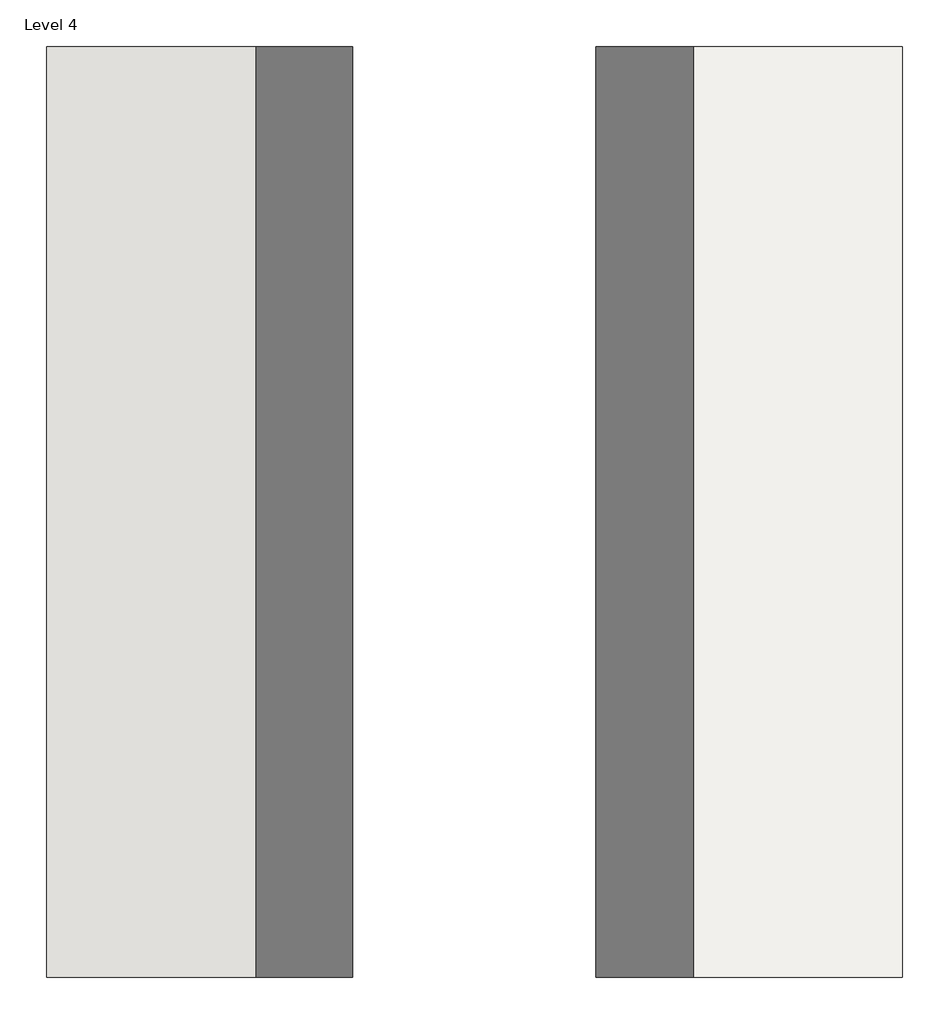
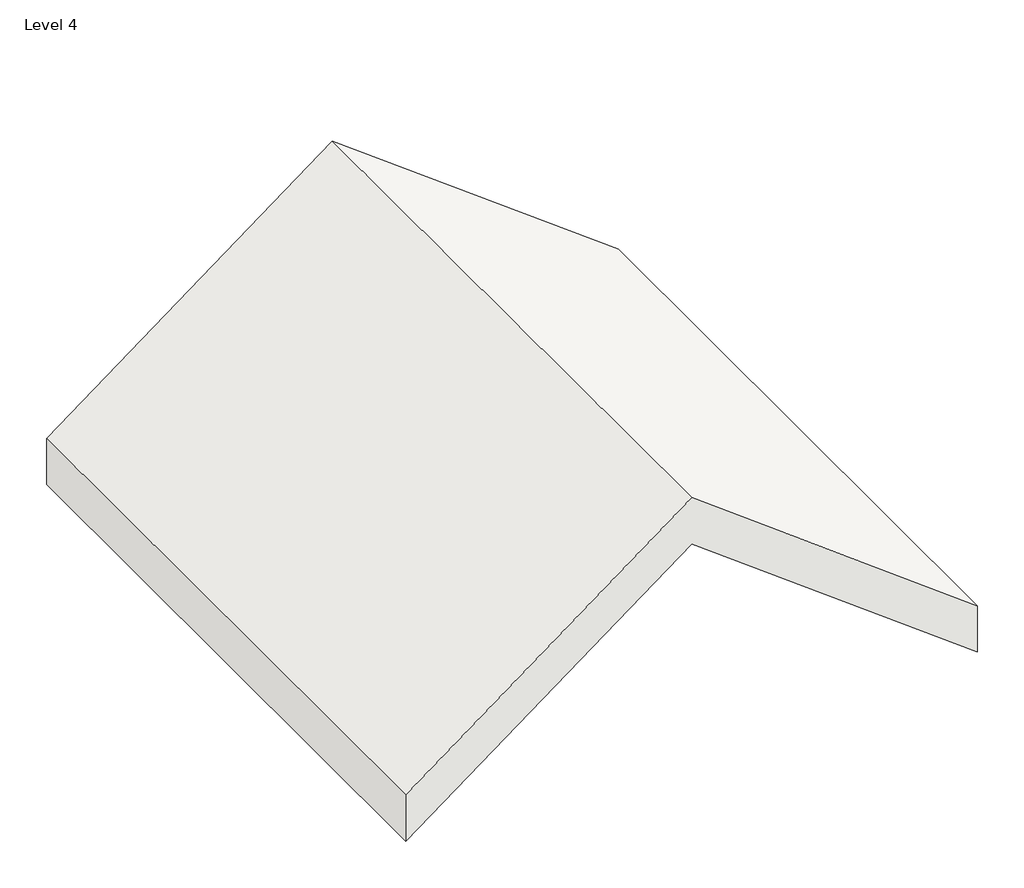
# One storey: 1 roof.
"""IFC4 building model written with IfcOpenShell, lengths in millimetres."""

from ifc_helpers import new_model, si_unit, frame, origin, place, context, project, spatial, polyline, outline, extrude, element, save

model = new_model("IFC4")

# Units and contexts
model_context = context("Model", 3, world=origin())
ifc_project = project(units=[si_unit("LENGTHUNIT", "METRE", prefix="MILLI")], contexts=[model_context])

# Site, building, storey
site = spatial("IfcSite", under=ifc_project)
building = spatial("IfcBuilding", under=site)
storey = spatial("IfcBuildingStorey", under=building, Name="Level 4", Elevation=6248.4)

# Roof
placement = place(None, origin())
element("IfcRoof", 1, ObjectType="Generic - 12\"", at=placement, inside=storey, context=model_context, shape_type="SweptSolid", body=[
    extrude(outline(polyline([(6629.4, 2524.7084887), (8305.8, 289.5084887), (6629.4, -1945.6915113), (6248.4, -1945.6915113), (7924.8, 289.5084887), (6248.4, 2524.7084887), (6629.4, 2524.7084887)])), frame((0.0, -245.2900369, 0.0), z_axis=(0.0, 1.0, 0.0), x_axis=(0.0, 0.0, 1.0)), (0.0, 0.0, 1.0), 4860.6702709),
])

save(model, "model.ifc")

# Revit data of these elements
# Type "Generic - 12\""
#   Assembly Code = "B1020"
# Element 1 (IfcRoof, "Generic - 12\"")
#   built-in parameter 1001705 = 27.25 (stored number, unit not read)
#   built-in parameter 1001710 = 33615
#   Phase Created = New Construction
